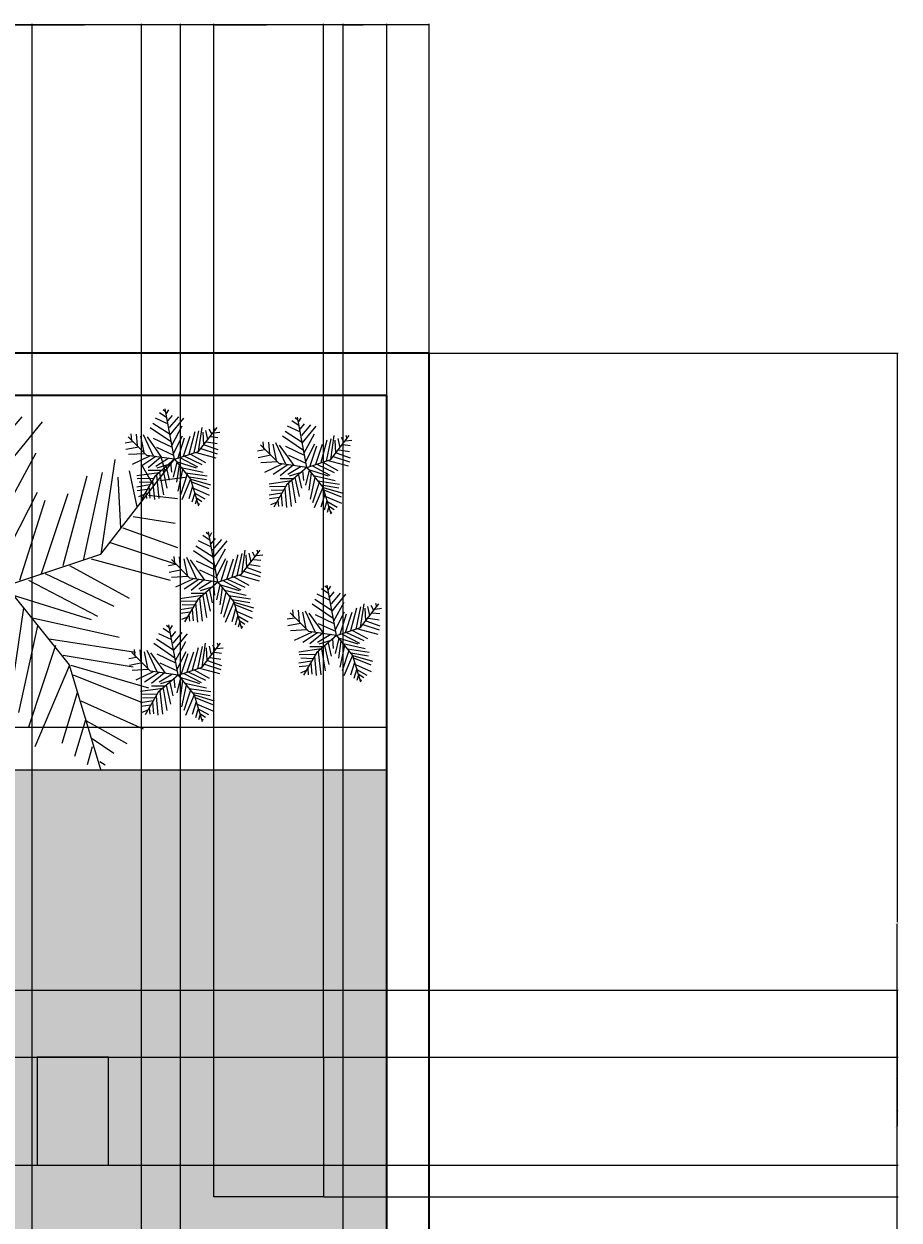
# Model space of a CAD drawing. Units: inches. Extents: x 818 to 1898, y 976 to 2364.
# Tile 96 of 96: x 1713 to 1898, y 2111 to 2364. Entities that reach past the tile are written whole.
import ezdxf

# ---------------------------------------------------------------- set-up
doc = ezdxf.new("R2010")
doc.units = ezdxf.units.IN
doc.header["$LTSCALE"] = 5
doc.header["$MEASUREMENT"] = 0
for name, color, linetype, lineweight in [('A-ANNO-DIMS', 2, 'Continuous', 18), ('C-PROP', 7, 'Continuous', 35), ('L-PAVE', 8, 'Continuous', 18), ('L-PLNT-BEDS', 94, 'Continuous', 18)]:
    doc.layers.add(name, color=color, linetype=linetype, lineweight=lineweight)
for name, color, linetype, lineweight, true_color in [('L-PAVE-PATT', 9, 'Continuous', 9, 0xc7c8ca), ('L-PLNT', 116, 'Continuous', 13, 0x136734), ('L-PLNT-PATT', 114, 'Continuous', 9, 0x139b48)]:
    doc.layers.add(name, color=color, linetype=linetype, lineweight=lineweight, true_color=true_color)
doc.styles.get("Standard").update_dxf_attribs({"font": 'arial.ttf'})
doc.dimstyles.get("Standard").update_dxf_attribs({"dimtxt": 0.18, "dimasz": 0.18, "dimexe": 0.18, "dimexo": 0.0625, "dimgap": 0.09, "dimtad": 0, "dimtih": 1, "dimtoh": 1, "dimdec": 4, "dimzin": 0, "dimdsep": 46, "dimtxsty": 'Standard', "dimcen": 0.09, "dimadec": 0, "dimazin": 0, "dimtfac": 1, "dimtdec": 4, "dimtofl": 0, "dimtmove": 0, "dimatfit": 3, "dimfxl": 1, "dimtolj": 1, "dimtzin": 0, "dimarcsym": 0})

# ---------------------------------------------------------------- blocks, each defined once
blk = doc.blocks.new('SHRUB-ACCENT')
for p, q in [((8.53, 19.84), (7.99, 20.28)), ((10.44, 9.82), (8.47, 20.47)), ((8.74, 19.5), (9.21, 20.28)), ((9.08, 17.24), (6.37, 18.54)), ((8.8, 18.63), (7.25, 19.67)), ((9.01, 17.93), (9.96, 19.06)), ((9.35, 16.54), (11.31, 18.8)), ((9.48, 14.98), (12.39, 18.54)), ((1.35, 13.77), (1.22, 15.24)), ((9.75, 13.42), (5.28, 16.46)), ((9.48, 15.07), (5.82, 17.41)), ((9.89, 12.9), (12.06, 16.89)), ((13.48, 10.9), (14.76, 15.68)), ((14.56, 11.16), (15.58, 15.85)), ((15.49, 11.5), (19.41, 16.55)), ((15.51, 11.51), (16.25, 16.54)), ((16.39, 15.59), (16.53, 12.9)), ((17, 15.94), (17.41, 14.03)), ((17.68, 16.2), (18.29, 15.16)), ((18.62, 15.42), (19.98, 15.59)), ((18.69, 16.63), (18.9, 15.94)), ((1.56, 13.51), (0, 13.25)), ((4.55, 10.66), (0.62, 14.58)), ((2.3, 15.16), (2.51, 12.72)), ((3.25, 14.72), (3.93, 11.25)), ((3.79, 15.07), (5.89, 10.55)), ((7.72, 10.21), (4.67, 14.55)), ((5.89, 14.29), (9.89, 12.38)), ((10.23, 11.07), (12.12, 14.81)), ((11.17, 10.12), (12.53, 14.37)), ((12.33, 10.47), (13.75, 14.72)), ((16.66, 12.9), (19.57, 11.86)), ((17.2, 13.51), (19.44, 13.16)), ((18.02, 14.63), (19.57, 14.46)), ((2.84, 12.38), (0.14, 11.86)), ((4.2, 10.99), (0.68, 10.81)), ((5.15, 10.47), (1.49, 8.73)), ((6.43, 10.38), (3.32, 8.3)), ((10.44, 9.82), (4.55, 10.66)), ((7.45, 10.21), (4.81, 8.04)), ((6.57, 12.38), (10.23, 10.73)), ((10.44, 9.82), (15.49, 11.5)), ((12.53, 10.47), (16.19, 8.73)), ((13.82, 10.9), (17, 9.16)), ((14.97, 11.25), (19.17, 10.12)), ((15.98, 12.12), (19.44, 10.99)), ((10.44, 9.82), (6.23, 6.17)), ((9.21, 10.03), (6.43, 8.3)), ((9.21, 8.73), (6.7, 7.95)), ((7.92, 7.69), (8.8, 3.69)), ((8.67, 8.21), (9.28, 5.43)), ((9.55, 9.16), (9.75, 7.08)), ((10.9, 9.25), (10.16, 6.04)), ((10.44, 9.82), (13.8, 5.61)), ((10.77, 9.34), (14.97, 8.04)), ((11.38, 8.64), (10.84, 5)), ((12.12, 7.69), (11.11, 3.09)), ((11.65, 10.12), (15.31, 8.21)), ((11.85, 8.12), (16.46, 7.08)), ((7.18, 6.99), (2.44, 6.3)), ((5.89, 5.78), (2.51, 5.69)), ((6.23, 6.17), (3.43, 1.4)), ((7.59, 7.43), (4.81, 7.43)), ((5.76, 5.34), (6.16, 1.35)), ((6.57, 6.39), (7.11, 1.52)), ((7.25, 6.99), (8.06, 2.31)), ((13.07, 6.65), (11.65, 2.31)), ((13.82, 5.6), (11.99, 1.26)), ((12.73, 6.99), (17.34, 6.3)), ((13.48, 6.13), (17.2, 5.52)), ((13.8, 5.61), (15.49, 0)), ((13.88, 5.6), (18.02, 4.39)), ((14.02, 5.08), (17.68, 3.61)), ((5.15, 4.39), (2.44, 3.95)), ((4.67, 3.43), (2.51, 3.17)), ((5.42, 4.91), (2.91, 5)), ((4.33, 2.91), (4.47, 1.52)), ((5.01, 4.04), (5.21, 1.61)), ((14.22, 4.13), (13.41, 1.44)), ((14.7, 2.74), (14.09, 0.74)), ((14.43, 3.69), (17.74, 2.22)), ((14.7, 2.65), (16.86, 1.44)), ((4, 2.39), (2.78, 1.87)), ((15.04, 1.26), (14.76, 0.31)), ((15.04, 1.7), (16.19, 0.92)), ((15.44, 0.48), (15.71, 0.31))]:
    blk.add_line(p, q)
blk = doc.blocks.new('PALM-BORDER')
for p, q in [((41.53, 39.05), (33.72, 81.45)), ((33.95, 78.95), (31.8, 80.68)), ((34.76, 77.57), (36.65, 80.68)), ((35.03, 74.11), (28.83, 78.26)), ((36.11, 68.59), (25.33, 73.77)), ((35.84, 71.35), (39.61, 75.84)), ((37.18, 65.82), (45, 74.8)), ((37.72, 59.6), (49.31, 73.77)), ((37.72, 59.95), (23.17, 69.28)), ((39.34, 51.31), (47.96, 67.2)), ((61.61, 45.75), (77.23, 65.83)), ((61.71, 45.79), (64.67, 65.82)), ((74.37, 66.17), (75.18, 63.4)), ((38.8, 53.39), (21.02, 65.48)), ((67.63, 63.4), (69.25, 55.81)), ((70.33, 64.44), (72.75, 60.3)), ((53.62, 43.37), (58.74, 62.37)), ((57.93, 44.41), (61.97, 63.06)), ((65.21, 62.02), (65.75, 51.31)), ((74.1, 61.33), (79.49, 62.02)), ((5.39, 54.77), (4.85, 60.64)), ((9.16, 60.3), (9.97, 50.62)), ((12.93, 58.57), (15.63, 44.75)), ((15.09, 59.95), (23.44, 41.99)), ((40.69, 44.06), (48.23, 58.91)), ((49.04, 41.64), (54.7, 58.57)), ((71.68, 58.22), (77.87, 57.53)), ((18.1, 42.4), (2.48, 58.02)), ((30.72, 40.61), (18.59, 57.88)), ((23.44, 56.84), (39.34, 49.24)), ((44.46, 40.26), (49.85, 57.19)), ((6.2, 53.73), (0, 52.7)), ((68.44, 53.73), (77.33, 52.35)), ((66.29, 51.31), (77.87, 47.17)), ((11.32, 49.24), (0.54, 47.17)), ((26.14, 49.24), (40.69, 42.68)), ((63.59, 48.21), (77.33, 43.71)), ((41.53, 39.05), (61.61, 45.75)), ((16.71, 43.71), (2.69, 43.02)), ((54.97, 43.37), (67.63, 36.46)), ((59.55, 44.75), (76.26, 40.26)), ((20.48, 41.64), (5.93, 34.73)), ((25.6, 41.3), (13.2, 33.01)), ((41.53, 39.05), (18.1, 42.4)), ((29.64, 40.61), (19.13, 31.97)), ((49.85, 41.64), (64.4, 34.73)), ((41.53, 39.05), (24.79, 24.55)), ((36.65, 39.91), (25.6, 33.01)), ((41.53, 39.05), (54.92, 22.32)), ((46.35, 40.26), (60.9, 32.66)), ((37.99, 36.46), (38.8, 28.17)), ((43.38, 36.81), (40.42, 24.02)), ((42.84, 37.15), (59.55, 31.97)), ((36.65, 34.73), (26.68, 31.62)), ((45.27, 34.39), (43.11, 19.88)), ((31.53, 30.59), (35.03, 14.7)), ((34.49, 32.66), (36.92, 21.61)), ((48.23, 30.59), (44.19, 12.28)), ((47.15, 32.32), (65.48, 28.17)), ((30.18, 29.55), (19.13, 29.55)), ((28.56, 27.82), (9.7, 25.06)), ((26.14, 25.41), (28.29, 6.06)), ((28.83, 27.82), (32.07, 9.17)), ((52, 26.44), (46.35, 9.17)), ((50.66, 27.82), (68.98, 25.06)), ((23.44, 22.99), (9.97, 22.64)), ((24.79, 24.55), (13.63, 5.58)), ((53.62, 24.37), (68.44, 21.95)), ((22.9, 21.26), (24.52, 5.37)), ((54.97, 22.3), (47.69, 5.02)), ((54.92, 22.32), (61.61, 0)), ((55.24, 22.3), (71.68, 17.46)), ((21.56, 19.53), (11.59, 19.88)), ((55.78, 20.22), (70.33, 14.35)), ((20.48, 17.46), (9.7, 15.73)), ((19.94, 16.08), (20.75, 6.41)), ((56.59, 16.42), (53.35, 5.72)), ((18.59, 13.66), (9.97, 12.62)), ((57.39, 14.7), (70.6, 8.83)), ((17.24, 11.59), (17.78, 6.06)), ((58.47, 10.9), (56.05, 2.95)), ((58.47, 10.55), (67.09, 5.72)), ((15.9, 9.52), (11.05, 7.44)), ((59.82, 6.75), (64.4, 3.64)), ((59.82, 5.02), (58.74, 1.22)), ((61.44, 1.92), (62.51, 1.22))]:
    blk.add_line(p, q)
blk = doc.blocks.new('*D57')
at = {"layer": 'A-ANNO-DIMS', "color": 0, "lineweight": -2, "ltscale": 5, "transparency": 16777216}
for p, q in [((992.73, 2294.28), (992.73, 2363.87)), ((992.91, 2363.69), (1395.43, 2363.69)), ((1798.54, 2363.69), (1396.01, 2363.69)), ((1798.72, 2294.28), (1798.72, 2363.87))]:
    blk.add_line(p, q, dxfattribs=at)
at = {"layer": 'A-ANNO-DIMS', "color": 0, "ltscale": 5, "transparency": 16777216}
for points in [[(992.91, 2363.72), (992.91, 2363.66), (992.73, 2363.69)], [(1798.54, 2363.72), (1798.54, 2363.66), (1798.72, 2363.69)]]:
    blk.add_solid(points, dxfattribs=at)
at = {"layer": 'Defpoints', "color": 0, "ltscale": 5, "transparency": 16777216}
for p in [(1798.72, 2363.69), (992.73, 2294.22), (1798.72, 2294.22)]:
    blk.add_point(p, dxfattribs=at)
at = {"layer": 'A-ANNO-DIMS', "color": 0, "ltscale": 5, "transparency": 16777216, "insert": (1395.72, 2363.69), "char_height": 0.18, "attachment_point": 5}
blk.add_mtext('\\A1;806', dxfattribs=at)
blk = doc.blocks.new('*D72')
at = {"layer": 'A-ANNO-DIMS', "color": 0, "lineweight": -2, "ltscale": 5, "transparency": 16777216}
for p, q in [((1798.78, 2294.22), (1897.92, 2294.22)), ((1897.74, 2294.04), (1897.74, 2173.83)), ((1897.74, 2053.26), (1897.74, 2173.47)), ((1714.79, 2053.08), (1897.92, 2053.08))]:
    blk.add_line(p, q, dxfattribs=at)
at = {"layer": 'A-ANNO-DIMS', "color": 0, "ltscale": 5, "transparency": 16777216}
for points in [[(1897.71, 2294.04), (1897.77, 2294.04), (1897.74, 2294.22)], [(1897.71, 2053.26), (1897.77, 2053.26), (1897.74, 2053.08)]]:
    blk.add_solid(points, dxfattribs=at)
at = {"layer": 'Defpoints', "color": 0, "ltscale": 5, "transparency": 16777216}
for p in [(1798.72, 2294.22), (1897.74, 2294.22), (1714.73, 2053.08)]:
    blk.add_point(p, dxfattribs=at)
at = {"layer": 'A-ANNO-DIMS', "color": 0, "ltscale": 5, "transparency": 16777216, "insert": (1897.74, 2173.65), "char_height": 0.18, "attachment_point": 5}
blk.add_mtext('\\A1;241.14', dxfattribs=at)
blk = doc.blocks.new('*D86')
at = {"layer": 'A-ANNO-DIMS', "color": 0, "lineweight": -2, "ltscale": 5, "transparency": 16777216}
for p, q in [((1258.73, 2053.14), (1258.73, 2363.87)), ((1258.91, 2363.69), (1486.43, 2363.69)), ((1714.55, 2363.69), (1487.02, 2363.69)), ((1714.73, 2053.14), (1714.73, 2363.87))]:
    blk.add_line(p, q, dxfattribs=at)
at = {"layer": 'A-ANNO-DIMS', "color": 0, "ltscale": 5, "transparency": 16777216}
for points in [[(1258.91, 2363.72), (1258.91, 2363.66), (1258.73, 2363.69)], [(1714.55, 2363.72), (1714.55, 2363.66), (1714.73, 2363.69)]]:
    blk.add_solid(points, dxfattribs=at)
at = {"layer": 'Defpoints', "color": 0, "ltscale": 5, "transparency": 16777216}
for p in [(1714.73, 2363.69), (1258.73, 2053.08), (1714.73, 2053.08)]:
    blk.add_point(p, dxfattribs=at)
at = {"layer": 'A-ANNO-DIMS', "color": 0, "ltscale": 5, "transparency": 16777216, "insert": (1486.73, 2363.69), "char_height": 0.18, "attachment_point": 5}
blk.add_mtext('\\A1;456', dxfattribs=at)
blk = doc.blocks.new('*D104')
at = {"layer": 'A-ANNO-DIMS', "color": 0, "lineweight": -2, "ltscale": 5, "transparency": 16777216}
for p, q in [((1689.47, 1071.12), (1689.47, 2363.87)), ((1689.65, 2363.69), (1717.4, 2363.69)), ((1745.9, 2363.69), (1718.15, 2363.69)), ((1746.08, 1071.12), (1746.08, 2363.87))]:
    blk.add_line(p, q, dxfattribs=at)
at = {"layer": 'A-ANNO-DIMS', "color": 0, "ltscale": 5, "transparency": 16777216}
for points in [[(1689.65, 2363.72), (1689.65, 2363.66), (1689.47, 2363.69)], [(1745.9, 2363.72), (1745.9, 2363.66), (1746.08, 2363.69)]]:
    blk.add_solid(points, dxfattribs=at)
at = {"layer": 'Defpoints', "color": 0, "ltscale": 5, "transparency": 16777216}
for p in [(1746.08, 2363.69), (1689.47, 1071.06), (1746.08, 1071.06)]:
    blk.add_point(p, dxfattribs=at)
at = {"layer": 'A-ANNO-DIMS', "color": 0, "ltscale": 5, "transparency": 16777216, "insert": (1717.78, 2363.69), "char_height": 0.18, "attachment_point": 5}
blk.add_mtext('\\A1;56.61', dxfattribs=at)
blk = doc.blocks.new('*D147')
at = {"layer": 'A-ANNO-DIMS', "color": 0, "lineweight": -2, "ltscale": 5, "transparency": 16777216}
for p, q in [((1212.58, 2145.25), (1897.92, 2145.25)), ((1897.74, 2145.07), (1897.74, 2133.99)), ((1897.74, 2122.56), (1897.74, 2133.63)), ((1212.58, 2122.38), (1897.92, 2122.38))]:
    blk.add_line(p, q, dxfattribs=at)
at = {"layer": 'A-ANNO-DIMS', "color": 0, "ltscale": 5, "transparency": 16777216}
for points in [[(1897.71, 2145.07), (1897.77, 2145.07), (1897.74, 2145.25)], [(1897.71, 2122.56), (1897.77, 2122.56), (1897.74, 2122.38)]]:
    blk.add_solid(points, dxfattribs=at)
at = {"layer": 'Defpoints', "color": 0, "ltscale": 5, "transparency": 16777216}
for p in [(1212.52, 2145.25), (1897.74, 2145.25), (1212.52, 2122.38)]:
    blk.add_point(p, dxfattribs=at)
at = {"layer": 'A-ANNO-DIMS', "color": 0, "ltscale": 5, "transparency": 16777216, "insert": (1897.74, 2133.81), "char_height": 0.18, "attachment_point": 5}
blk.add_mtext('\\A1;22.87', dxfattribs=at)
blk = doc.blocks.new('*D148')
at = {"layer": 'A-ANNO-DIMS', "color": 0, "lineweight": -2, "ltscale": 5, "transparency": 16777216}
for p, q in [((1232.67, 2159.43), (1897.92, 2159.43)), ((1897.74, 2159.25), (1897.74, 2141.09)), ((1897.74, 2122.56), (1897.74, 2140.72)), ((1232.67, 2122.38), (1897.92, 2122.38))]:
    blk.add_line(p, q, dxfattribs=at)
at = {"layer": 'A-ANNO-DIMS', "color": 0, "ltscale": 5, "transparency": 16777216}
for points in [[(1897.71, 2159.25), (1897.77, 2159.25), (1897.74, 2159.43)], [(1897.71, 2122.56), (1897.77, 2122.56), (1897.74, 2122.38)]]:
    blk.add_solid(points, dxfattribs=at)
at = {"layer": 'Defpoints', "color": 0, "ltscale": 5, "transparency": 16777216}
for p in [(1232.61, 2159.43), (1897.74, 2159.43), (1232.61, 2122.38)]:
    blk.add_point(p, dxfattribs=at)
at = {"layer": 'A-ANNO-DIMS', "color": 0, "ltscale": 5, "transparency": 16777216, "insert": (1897.74, 2140.9), "char_height": 0.18, "attachment_point": 5}
blk.add_mtext('\\A1;37.05', dxfattribs=at)
blk = doc.blocks.new('*D149')
at = {"layer": 'A-ANNO-DIMS', "color": 0, "lineweight": -2, "ltscale": 5, "transparency": 16777216}
for p, q in [((1753.17, 2115.75), (1753.17, 2363.87)), ((1753.35, 2363.69), (1764.28, 2363.69)), ((1776.15, 2363.69), (1765.21, 2363.69)), ((1776.33, 2145.31), (1776.33, 2363.87))]:
    blk.add_line(p, q, dxfattribs=at)
at = {"layer": 'A-ANNO-DIMS', "color": 0, "ltscale": 5, "transparency": 16777216}
for points in [[(1753.35, 2363.72), (1753.35, 2363.66), (1753.17, 2363.69)], [(1776.15, 2363.72), (1776.15, 2363.66), (1776.33, 2363.69)]]:
    blk.add_solid(points, dxfattribs=at)
at = {"layer": 'Defpoints', "color": 0, "ltscale": 5, "transparency": 16777216}
for p in [(1776.33, 2363.69), (1776.33, 2145.25), (1753.17, 2115.69)]:
    blk.add_point(p, dxfattribs=at)
at = {"layer": 'A-ANNO-DIMS', "color": 0, "ltscale": 5, "transparency": 16777216, "insert": (1764.75, 2363.69), "char_height": 0.18, "attachment_point": 5}
blk.add_mtext('\\A1;23.166', dxfattribs=at)
blk = doc.blocks.new('*D150')
at = {"layer": 'A-ANNO-DIMS', "color": 0, "lineweight": -2, "ltscale": 5, "transparency": 16777216}
for p, q in [((1776.39, 2145.25), (1897.92, 2145.25)), ((1897.74, 2145.07), (1897.74, 2130.65)), ((1897.74, 2115.87), (1897.74, 2130.29)), ((1776.39, 2115.69), (1897.92, 2115.69))]:
    blk.add_line(p, q, dxfattribs=at)
at = {"layer": 'A-ANNO-DIMS', "color": 0, "ltscale": 5, "transparency": 16777216}
for points in [[(1897.71, 2145.07), (1897.77, 2145.07), (1897.74, 2145.25)], [(1897.71, 2115.87), (1897.77, 2115.87), (1897.74, 2115.69)]]:
    blk.add_solid(points, dxfattribs=at)
at = {"layer": 'Defpoints', "color": 0, "ltscale": 5, "transparency": 16777216}
for p in [(1776.33, 2145.25), (1897.74, 2145.25), (1776.33, 2115.69)]:
    blk.add_point(p, dxfattribs=at)
at = {"layer": 'A-ANNO-DIMS', "color": 0, "ltscale": 5, "transparency": 16777216, "insert": (1897.74, 2130.47), "char_height": 0.18, "attachment_point": 5}
blk.add_mtext('\\A1;29.557', dxfattribs=at)
blk = doc.blocks.new('*D186')
at = {"layer": 'A-ANNO-DIMS', "color": 0, "lineweight": -2, "ltscale": 5, "transparency": 16777216}
for p, q in [((1714.73, 1549.14), (1714.73, 2363.87)), ((1714.91, 2363.69), (1725.82, 2363.69)), ((1737.66, 2363.69), (1726.75, 2363.69)), ((1737.84, 1549.14), (1737.84, 2363.87))]:
    blk.add_line(p, q, dxfattribs=at)
at = {"layer": 'A-ANNO-DIMS', "color": 0, "ltscale": 5, "transparency": 16777216}
for points in [[(1714.91, 2363.72), (1714.91, 2363.66), (1714.73, 2363.69)], [(1737.66, 2363.72), (1737.66, 2363.66), (1737.84, 2363.69)]]:
    blk.add_solid(points, dxfattribs=at)
at = {"layer": 'Defpoints', "color": 0, "ltscale": 5, "transparency": 16777216}
for p in [(1737.84, 2363.69), (1714.73, 1549.08), (1737.84, 1549.08)]:
    blk.add_point(p, dxfattribs=at)
at = {"layer": 'A-ANNO-DIMS', "color": 0, "ltscale": 5, "transparency": 16777216, "insert": (1726.28, 2363.69), "char_height": 0.18, "attachment_point": 5}
blk.add_mtext('\\A1;23.116', dxfattribs=at)
blk = doc.blocks.new('*D205')
at = {"layer": 'A-ANNO-DIMS', "color": 0, "lineweight": -2, "ltscale": 5, "transparency": 16777216}
for p, q in [((1590.73, 2044.14), (1590.73, 2363.87)), ((1590.91, 2363.69), (1652.45, 2363.69)), ((1714.55, 2363.69), (1653.01, 2363.69)), ((1714.73, 2053.14), (1714.73, 2363.87))]:
    blk.add_line(p, q, dxfattribs=at)
at = {"layer": 'A-ANNO-DIMS', "color": 0, "ltscale": 5, "transparency": 16777216}
for points in [[(1590.91, 2363.72), (1590.91, 2363.66), (1590.73, 2363.69)], [(1714.55, 2363.72), (1714.55, 2363.66), (1714.73, 2363.69)]]:
    blk.add_solid(points, dxfattribs=at)
at = {"layer": 'Defpoints', "color": 0, "ltscale": 5, "transparency": 16777216}
for p in [(1714.73, 2363.69), (1714.73, 2053.08), (1590.73, 2044.08)]:
    blk.add_point(p, dxfattribs=at)
at = {"layer": 'A-ANNO-DIMS', "color": 0, "ltscale": 5, "transparency": 16777216, "insert": (1652.73, 2363.69), "char_height": 0.18, "attachment_point": 5}
blk.add_mtext('\\A1;124', dxfattribs=at)
blk = doc.blocks.new('*D262')
at = {"layer": 'A-ANNO-DIMS', "color": 0, "lineweight": -2, "ltscale": 5, "transparency": 16777216}
for p, q in [((1714.73, 1957.1), (1714.73, 2363.87)), ((1714.91, 2363.69), (1725.82, 2363.69)), ((1737.66, 2363.69), (1726.75, 2363.69)), ((1737.84, 1957.1), (1737.84, 2363.87))]:
    blk.add_line(p, q, dxfattribs=at)
at = {"layer": 'A-ANNO-DIMS', "color": 0, "ltscale": 5, "transparency": 16777216}
for points in [[(1714.91, 2363.72), (1714.91, 2363.66), (1714.73, 2363.69)], [(1737.66, 2363.72), (1737.66, 2363.66), (1737.84, 2363.69)]]:
    blk.add_solid(points, dxfattribs=at)
at = {"layer": 'Defpoints', "color": 0, "ltscale": 5, "transparency": 16777216}
for p in [(1737.84, 2363.69), (1714.73, 1957.03), (1737.84, 1957.03)]:
    blk.add_point(p, dxfattribs=at)
at = {"layer": 'A-ANNO-DIMS', "color": 0, "ltscale": 5, "transparency": 16777216, "insert": (1726.28, 2363.69), "char_height": 0.18, "attachment_point": 5}
blk.add_mtext('\\A1;23.116', dxfattribs=at)
blk = doc.blocks.new('*D265')
at = {"layer": 'A-ANNO-DIMS', "color": 0, "lineweight": -2, "ltscale": 5, "transparency": 16777216}
for p, q in [((1780.5, 2053.14), (1780.5, 2363.87)), ((1780.68, 2363.69), (1784.72, 2363.69)), ((1789.54, 2363.69), (1785.5, 2363.69)), ((1789.72, 2053.14), (1789.72, 2363.87))]:
    blk.add_line(p, q, dxfattribs=at)
at = {"layer": 'A-ANNO-DIMS', "color": 0, "ltscale": 5, "transparency": 16777216}
for points in [[(1780.68, 2363.72), (1780.68, 2363.66), (1780.5, 2363.69)], [(1789.54, 2363.72), (1789.54, 2363.66), (1789.72, 2363.69)]]:
    blk.add_solid(points, dxfattribs=at)
at = {"layer": 'Defpoints', "color": 0, "ltscale": 5, "transparency": 16777216}
for p in [(1789.72, 2363.69), (1780.5, 2053.08), (1789.72, 2053.08)]:
    blk.add_point(p, dxfattribs=at)
at = {"layer": 'A-ANNO-DIMS', "color": 0, "ltscale": 5, "transparency": 16777216, "insert": (1785.11, 2363.69), "char_height": 0.18, "attachment_point": 5}
blk.add_mtext('\\A1;9.215', dxfattribs=at)

msp = doc.modelspace()

# ---------------------------------------------------------------- hatches: boundary and pattern name
at = {"layer": 'L-PAVE-PATT', "ltscale": 5}
h = msp.add_hatch(color=256, dxfattribs=at)
h.dxf.hatch_style = 1
h.paths.add_polyline_path([(1212.5206, 2145.2461), (1197.3925, 2145.2461), (1197.3925, 2122.3767), (1212.5206, 2122.3767)])
h.paths.add_polyline_path([(1247.7373, 2159.4296), (1232.6091, 2159.4296), (1232.6091, 2122.3767), (1247.7373, 2122.3767)])
h.paths.add_polyline_path([(1282.9539, 2145.2461), (1267.8258, 2145.2461), (1267.8258, 2122.3767), (1282.9539, 2122.3767)])
h.paths.add_polyline_path([(1318.1705, 2145.2461), (1303.0424, 2145.2461), (1303.0424, 2122.3767), (1318.1705, 2122.3767)])
h.paths.add_polyline_path([(1353.3871, 2155.7839), (1338.259, 2155.7839), (1338.259, 2122.3767), (1353.3871, 2122.3767)])
h.paths.add_polyline_path([(1388.6037, 2145.2461), (1373.4756, 2145.2461), (1373.4756, 2122.3767), (1388.6037, 2122.3767)])
h.paths.add_polyline_path([(1423.8203, 2145.2461), (1408.6922, 2145.2461), (1408.6922, 2122.3767), (1423.8203, 2122.3767)])
h.paths.add_polyline_path([(1459.037, 2158.4222), (1443.9089, 2158.4222), (1443.9089, 2122.3767), (1459.037, 2122.3767)])
h.paths.add_polyline_path([(1494.2536, 2145.2461), (1479.1255, 2145.2461), (1479.1255, 2122.3767), (1494.2536, 2122.3767)])
h.paths.add_polyline_path([(1529.4702, 2145.2461), (1514.3421, 2145.2461), (1514.3421, 2122.3767), (1529.4702, 2122.3767)])
h.paths.add_polyline_path([(1564.6868, 2156.9246), (1549.5587, 2156.9246), (1549.5587, 2122.3767), (1564.6868, 2122.3767)])
h.paths.add_polyline_path([(1599.9034, 2145.2461), (1584.7753, 2145.2461), (1584.7753, 2122.3767), (1599.9034, 2122.3767)])
h.paths.add_polyline_path([(1635.1201, 2145.2461), (1619.9919, 2145.2461), (1619.9919, 2122.3767), (1635.1201, 2122.3767)])
h.paths.add_polyline_path([(1670.3367, 2156.1761), (1655.2086, 2156.1761), (1655.2086, 2122.3767), (1670.3367, 2122.3767)])
h.paths.add_polyline_path([(1701.7273, 2145.2461), (1686.5992, 2145.2461), (1686.5992, 2122.3767), (1701.7273, 2122.3767)])
h.paths.add_polyline_path([(1730.8897, 2145.2461), (1715.7616, 2145.2461), (1715.7616, 2122.3767), (1730.8897, 2122.3767)])
h.paths.add_polyline_path([(1776.3312, 2145.2461), (1753.1652, 2145.2461), (1753.1652, 2115.6891), (1776.3312, 2115.6891)])
at = {"layer": 'L-PLNT-PATT', "ltscale": 5}
h = msp.add_hatch(color=256, dxfattribs=at)
h.dxf.hatch_style = 1
h.paths.add_polyline_path([(1789.7173, 2205.9709), (1083.7252, 2205.9709), (1083.7252, 2083.2623), (1218.1114, 2083.2623), (1218.1114, 2053.0782), (1390.6356, 2053.0782), (1390.6356, 2081.1881), (1399.6356, 2081.1881), (1413.02, 2081.1881), (1422.02, 2081.1881), (1422.02, 2053.0782), (1676.6446, 2053.0782), (1676.6446, 2081.1881), (1714.7251, 2081.1881), (1714.7251, 2081.6235), (1789.7173, 2081.6235)])
h.paths.add_polyline_path([(1388.6037, 2145.2461), (1388.6037, 2122.3767), (1373.4756, 2122.3767), (1373.4756, 2145.2461)], flags=16)
h.paths.add_polyline_path([(1408.6922, 2145.2461), (1423.8203, 2145.2461), (1423.8203, 2122.3767), (1408.6922, 2122.3767)], flags=16)
h.paths.add_polyline_path([(1353.3871, 2155.7839), (1353.3871, 2122.3767), (1338.259, 2122.3767), (1338.259, 2155.7839)], flags=16)
h.paths.add_polyline_path([(1443.9089, 2158.4222), (1459.037, 2158.4222), (1459.037, 2122.3767), (1443.9089, 2122.3767)], flags=16)
h.paths.add_polyline_path([(1318.1705, 2145.2461), (1318.1705, 2122.3767), (1303.0424, 2122.3767), (1303.0424, 2145.2461)], flags=16)
h.paths.add_polyline_path([(1479.1255, 2145.2461), (1494.2536, 2145.2461), (1494.2536, 2122.3767), (1479.1255, 2122.3767)], flags=16)
h.paths.add_polyline_path([(1282.9539, 2145.2461), (1282.9539, 2122.3767), (1267.8258, 2122.3767), (1267.8258, 2145.2461)], flags=16)
h.paths.add_polyline_path([(1514.3421, 2145.2461), (1529.4702, 2145.2461), (1529.4702, 2122.3767), (1514.3421, 2122.3767)], flags=16)
h.paths.add_polyline_path([(1247.7373, 2159.4296), (1247.7373, 2122.3767), (1232.6091, 2122.3767), (1232.6091, 2159.4296)], flags=16)
h.paths.add_polyline_path([(1549.5587, 2156.9246), (1564.6868, 2156.9246), (1564.6868, 2122.3767), (1549.5587, 2122.3767)], flags=16)
h.paths.add_polyline_path([(1212.5206, 2145.2461), (1212.5206, 2122.3767), (1197.3925, 2122.3767), (1197.3925, 2145.2461)], flags=16)
h.paths.add_polyline_path([(1584.7753, 2145.2461), (1599.9034, 2145.2461), (1599.9034, 2122.3767), (1584.7753, 2122.3767)], flags=16)
h.paths.add_polyline_path([(1185.1073, 2104.7786), (1190.6407, 2104.7786), (1185.1073, 2098.2505), (1179.5738, 2104.7786)], flags=16)
h.paths.add_polyline_path([(1619.9919, 2145.2461), (1635.1201, 2145.2461), (1635.1201, 2122.3767), (1619.9919, 2122.3767)], flags=16)
h.paths.add_polyline_path([(1655.2086, 2156.1761), (1670.3367, 2156.1761), (1670.3367, 2122.3767), (1655.2086, 2122.3767)], flags=16)
h.paths.add_polyline_path([(1686.5992, 2145.2461), (1701.7273, 2145.2461), (1701.7273, 2122.3767), (1686.5992, 2122.3767)], flags=16)
h.paths.add_polyline_path([(1715.7616, 2145.2461), (1730.8897, 2145.2461), (1730.8897, 2122.3767), (1715.7616, 2122.3767)], flags=16)
h.paths.add_polyline_path([(1753.1652, 2145.2461), (1776.3312, 2145.2461), (1776.3312, 2115.6891), (1753.1652, 2115.6891)], flags=16)
h.paths.add_polyline_path([(1191.4331, 2146.5159), (1176.7891, 2146.5159), (1176.7891, 2134.1516), (1191.4331, 2134.1516)], flags=24)

# ---------------------------------------------------------------- linework, layer by layer
at = {"layer": 'C-PROP', "ltscale": 5}
for p, q in [((1798.7173, 2294.2171), (992.7251, 2294.2171)), ((1798.7173, 1202.9642), (1798.7173, 2294.2171)), ((1789.7173, 2285.2171), (1001.7252, 2285.2171)), ((1789.7173, 1211.9642), (1789.7173, 2285.2171))]:
    msp.add_line(p, q, dxfattribs=at)
at = {"layer": 'L-PAVE', "ltscale": 5}
for points in [[(1730.8897, 2145.2461), (1715.7616, 2145.2461), (1715.7616, 2122.3767), (1730.8897, 2122.3767)], [(1776.3312, 2115.6891), (1753.1652, 2115.6891), (1753.1652, 2145.2461), (1776.3312, 2145.2461)]]:
    msp.add_lwpolyline(points, close=True, dxfattribs=at)
at = {"layer": 'L-PLNT-BEDS', "ltscale": 5}
for p, q in [((1789.7173, 2214.9709), (1071.7252, 2214.9709)), ((1789.7173, 2205.9709), (1083.7252, 2205.9709))]:
    msp.add_line(p, q, dxfattribs=at)

# ---------------------------------------------------------------- block references
at = {"layer": 'L-PLNT'}
for name, p in [('PALM-BORDER', (1667.6244, 2205.9177)), ('SHRUB-ACCENT', (1734.418, 2261.9311)), ('SHRUB-ACCENT', (1762.389, 2260.2195)), ('SHRUB-ACCENT', (1743.5453, 2235.9519)), ('SHRUB-ACCENT', (1768.6703, 2224.6549)), ('SHRUB-ACCENT', (1735.1703, 2216.2868))]:
    msp.add_blockref(name, p, dxfattribs=at)

# ---------------------------------------------------------------- dimensions: what is measured, and where the dimension line sits
at = {"layer": 'A-ANNO-DIMS', "ltscale": 5}
for base, p1, p2, override, picture, middle in [((1798.7173, 2363.6929), (992.7251, 2294.2171), (1798.7173, 2294.2171), {"dimdec": 0, "dimlfac": 1, "dimrnd": 0, "dimzin": 0, "dimdsep": 46, "dimlunit": 2}, '*D57', (1395.7212, 2363.6929)), ((1714.7251, 2363.6929), (1258.7251, 2053.0782), (1714.7251, 2053.0782), {"dimdec": 0, "dimlfac": 1, "dimrnd": 0, "dimzin": 0, "dimdsep": 46, "dimlunit": 2}, '*D86', (1486.7251, 2363.6929)), ((1714.7251, 2363.6929), (1590.7251, 2044.0782), (1714.7251, 2053.0782), {"dimdec": 0, "dimlfac": 1, "dimrnd": 0, "dimzin": 0, "dimdsep": 46, "dimlunit": 2}, '*D205', (1652.7251, 2363.6929)), ((1746.0831, 2363.6929), (1689.4714, 1071.0552), (1746.0831, 1071.0552), {"dimdec": 2, "dimlfac": 1, "dimrnd": 0, "dimzin": 0, "dimdsep": 46, "dimlunit": 2}, '*D104', (1717.7772, 2363.6929)), ((1737.8409, 2363.6929), (1714.7251, 1549.0782), (1737.8409, 1549.0782), {"dimdec": 3, "dimlfac": 1, "dimrnd": 0, "dimzin": 0, "dimdsep": 46, "dimlunit": 2}, '*D186', (1726.283, 2363.6929)), ((1737.8409, 2363.6929), (1714.7251, 1957.0338), (1737.8409, 1957.0338), {"dimdec": 3, "dimlfac": 1, "dimrnd": 0, "dimzin": 0, "dimdsep": 46, "dimlunit": 2}, '*D262', (1726.283, 2363.6929)), ((1776.3312, 2363.6929), (1753.1652, 2115.6891), (1776.3312, 2145.2461), {"dimdec": 3, "dimlfac": 1, "dimrnd": 0, "dimzin": 0, "dimdsep": 46, "dimlunit": 2}, '*D149', (1764.7482, 2363.6929)), ((1789.7173, 2363.6929), (1780.5019, 2053.0782), (1789.7173, 2053.0782), {"dimdec": 3, "dimlfac": 1, "dimrnd": 0, "dimzin": 0, "dimdsep": 46, "dimlunit": 2}, '*D265', (1785.1096, 2363.6929))]:
    dim = msp.add_linear_dim(base=base, p1=p1, p2=p2, dimstyle='Standard', override=override, dxfattribs=at)
    dim.commit()
    dim.dimension.update_dxf_attribs({"geometry": picture, "text_midpoint": middle})
for base, p1, p2, override, picture, middle in [((1897.736, 2294.2171), (1714.7251, 2053.0782), (1798.7173, 2294.2171), {"dimdec": 2, "dimlfac": 1, "dimrnd": 0, "dimzin": 0, "dimdsep": 46, "dimlunit": 2}, '*D72', (1897.736, 2173.6477)), ((1897.736, 2159.4296), (1232.6091, 2122.3767), (1232.6091, 2159.4296), {"dimdec": 2, "dimlfac": 1, "dimrnd": 0, "dimzin": 0, "dimdsep": 46, "dimlunit": 2}, '*D148', (1897.736, 2140.9032)), ((1897.736, 2145.2461), (1212.5206, 2122.3767), (1212.5206, 2145.2461), {"dimdec": 2, "dimlfac": 1, "dimrnd": 0, "dimzin": 0, "dimdsep": 46, "dimlunit": 2}, '*D147', (1897.736, 2133.8114)), ((1897.736, 2145.2461), (1776.3312, 2115.6891), (1776.3312, 2145.2461), {"dimdec": 3, "dimlfac": 1, "dimrnd": 0, "dimzin": 0, "dimdsep": 46, "dimlunit": 2}, '*D150', (1897.736, 2130.4676))]:
    dim = msp.add_linear_dim(base=base, p1=p1, p2=p2, angle=90, dimstyle='Standard', override=override, dxfattribs=at)
    dim.commit()
    dim.dimension.update_dxf_attribs({"geometry": picture, "text_midpoint": middle})

doc.saveas('drawing.dxf')
